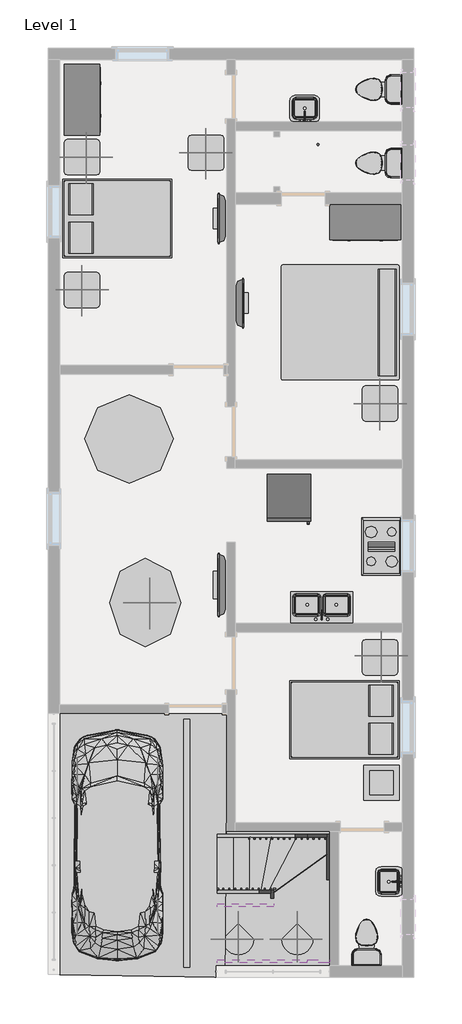
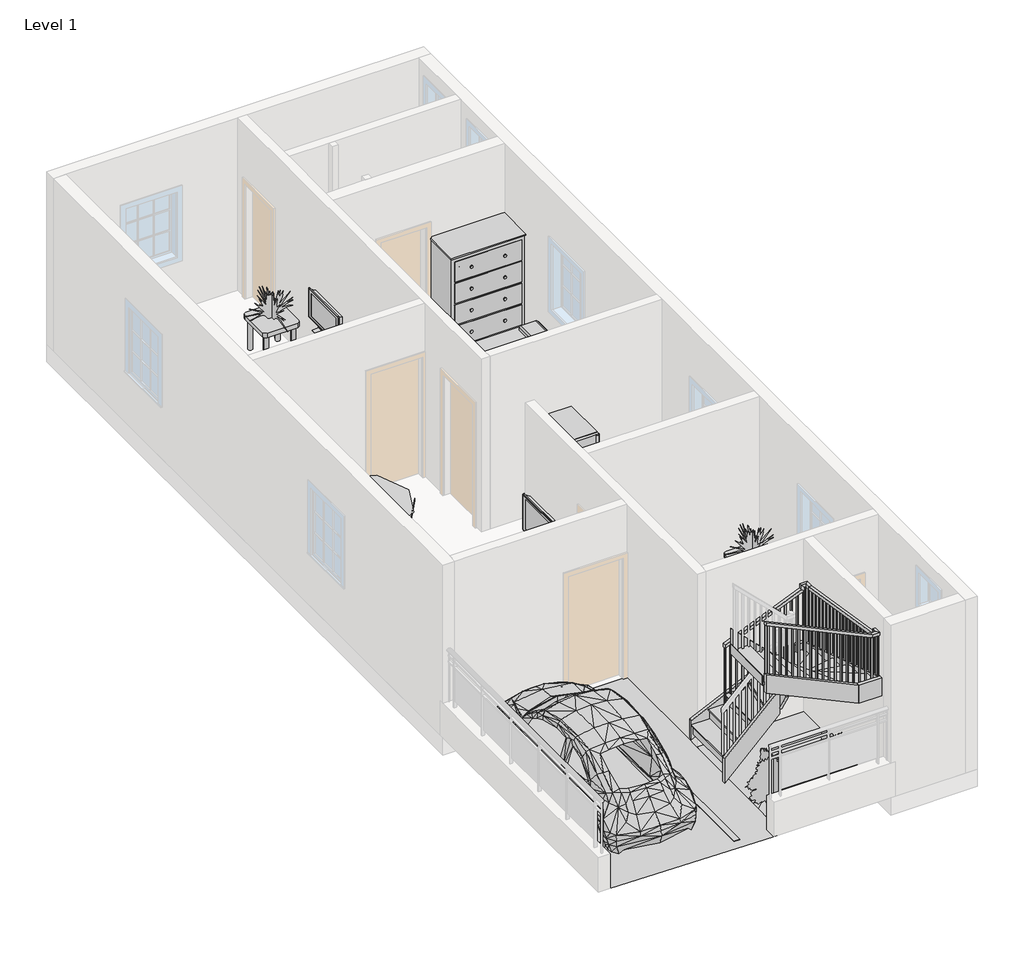
# One storey, part 3 of 3: 16 furniture elements, 10 flow terminals, 8 geographic elements, 8 members, 6 proxies, 1 railing, 1 stair flight.
# Revit data of these elements (continued)
# Element 25 (IfcFurniture, "Table-Coffee : 24\" x 24\" x 24\"") (continued)
#   Materials on its faces: "Glass - Clear, Grey"
# Element 26 (IfcFurniture, "Table-Dining Round w Chairs : 60\" Diameter")
#   Phase Created = New Construction
#   Materials on its faces: "Pine", "Laminate, Linen, Matte"
# Element 27 (IfcFurniture, "Table-Ellipse : 60\" x 48\"")
#   Phase Created = New Construction
#   Materials on its faces: "Birch"
# Elements 28, 29, 30, 31, 32 (IfcFurniture, "Table-End : 24\" x 24\"")
#   Phase Created = New Construction
#   Materials on its faces: "Laminate, Ivory, Matte", "Birch"
# Elements 33, 34, 35, 36, 37, 38 (IfcGeographicElement, "RPC Plant - Tropical : Agave - 1.5'")
#   Phase Created = New Construction
# Elements 39, 40 (IfcGeographicElement, "RPC Plant - Tropical : Jungle Flame - 3'")
#   Phase Created = New Construction
# Elements 41, 42, 43, 44, 45, 46, 47, 48 (IfcMember, "Stringer - 2\" Width")
#   Phase Created = New Construction
# Element 49 (IfcRailing, "Handrail - Rectangular")
#   Phase Created = New Construction
# Element 50 (IfcStairFlight, "2\" Tread 1\" Nosing 1/4\" Riser")
#   Phase Created = New Construction
# Materials
#   "Steel, Chrome Plated": class "Metal", colour RGB 17 17 17, transparency 0, Description = "Chromiuim plated steel", Cost = 0
#   "Steel, Polished": class "Metal", colour RGB 57 57 57, transparency 0, Description = "Polished steel", Cost = 0
#   "Steel, Paint Finish, Ivory, Glossy": class "Metal", colour RGB 247 247 239, transparency 0, Description = "Steel, paint finish, ivory, glossy", Cost = 0
#   "Porcelain, Linen": class "Ceramic", colour RGB 249 239 230, transparency 0, Description = "Porcelain, linen", Cost = 0
#   "Laminate, Linen, Matte": class "Plastic", colour RGB 249 239 230, transparency 0, Description = "Plastic Laminate - Linen, Matte", Cost = 0
#   "Birch": class "Wood", colour RGB 224 178 126, transparency 0, Description = "Betula Alleghaniensis", Cost = 0
#   "Linen, White": class "Textile", colour RGB 247 247 239, transparency 0, Description = "Linen, white", Cost = 0
#   "Laminate - Ivory, Glossy": colour RGB 247 247 239, transparency 0
#   "Laminate, Ivory, Matte": class "Plastic", colour RGB 247 247 239, transparency 0, Description = "Plastic Laminate - Ivory, Matte", Cost = 0
#   "Cherry": class "Wood", colour RGB 226 177 128, transparency 0, Description = "Prunus Serotina", Cost = 0
#   "Pine": class "Wood", colour RGB 223 192 134, transparency 0, Description = "Pinus Echinata", Cost = 0
#   "Parking Stripe": class "Paint", colour RGB 250 250 91, transparency 0
#   "TV - Black": colour RGB 49 49 49, transparency 0
#   "TV - Glass": colour RGB 157 157 157, transparency 0.9
#   "TV - Screen": colour RGB 0 0 0, transparency 0
#   "Glass - Clear, Grey": class "Glass", colour RGB 252 255 255, transparency 0.64
